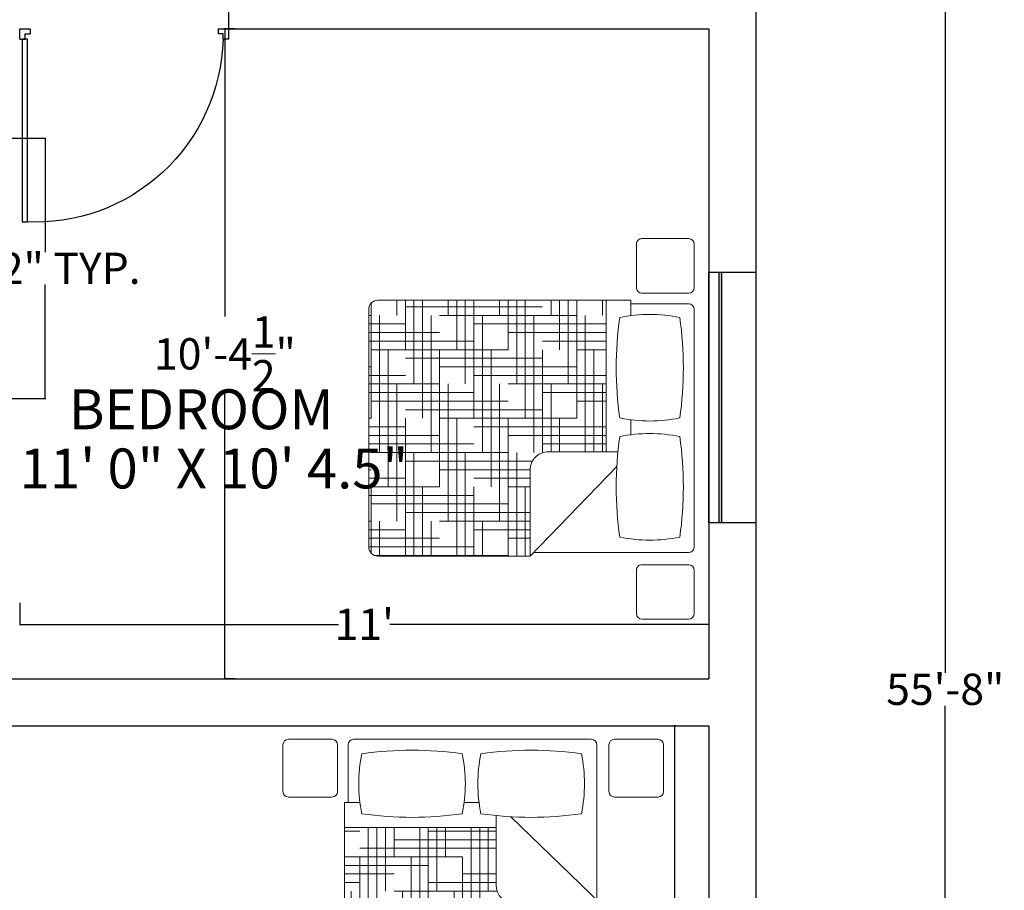
# Model space of a CAD drawing. Units: inches. Extents: x -113 to 5399, y -1393 to 3302.
# Tile 29 of 40: x 3982 to 4170, y 189 to 356. Entities that reach past the tile are written whole.
import ezdxf

# ---------------------------------------------------------------- set-up
doc = ezdxf.new("R2010")
doc.units = ezdxf.units.IN
doc.header["$MEASUREMENT"] = 0
for name, color, linetype, lineweight in [('A-ANNO-DIMS', 254, 'Continuous', 18), ('A-AREA-IDEN', 4, 'Continuous', 18), ('doors', 2, 'Continuous', 25), ('furniture', 131, 'Continuous', 18), ('walls', 1, 'Continuous', 25), ('windows', 3, 'Continuous', 25)]:
    doc.layers.add(name, color=color, linetype=linetype, lineweight=lineweight)
doc.styles.get("Standard").update_dxf_attribs({"font": 'arial.ttf'})
doc.dimstyles.get("Standard").update_dxf_attribs({"dimtxt": 6, "dimasz": 0.18, "dimexe": 0.18, "dimexo": 0.0625, "dimgap": 0.09, "dimtad": 0, "dimtih": 1, "dimtoh": 1, "dimdec": 1, "dimzin": 0, "dimdsep": 46, "dimlunit": 4, "dimtxsty": 'Standard', "dimblk": 'ARCHTICK', "dimcen": 0.09, "dimadec": 0, "dimazin": 0, "dimtfac": 1, "dimtdec": 1, "dimtofl": 0, "dimtmove": 0, "dimatfit": 3, "dimfxl": 1, "dimtolj": 1, "dimtzin": 0, "dimarcsym": 0})

# ---------------------------------------------------------------- blocks, each defined once
blk = doc.blocks.new('*X4')
at = {"color": 0}
for p, q in [((4.3594, 18.5625), (4.3594, 18.6457)), ((4.5, 18), (4.5, 18.6457)), ((4.5469, 18.1875), (4.5469, 18.6457)), ((4.5938, 18.375), (4.5938, 18.6457)), ((4.6406, 18.5625), (4.6406, 18.6457)), ((4.7812, 18), (4.7812, 18.6457)), ((4.8281, 18.1875), (4.8281, 18.6457)), ((4.875, 18.375), (4.875, 18.6457)), ((4.9219, 18.5625), (4.9219, 18.6457)), ((5.0625, 18), (5.0625, 18.6457)), ((5.1094, 18.1875), (5.1094, 18.6457)), ((5.1562, 18.375), (5.1562, 18.6457)), ((5.2031, 18.5625), (5.2031, 18.6457)), ((5.3438, 18), (5.3438, 18.6457)), ((5.3906, 18.1875), (5.3906, 18.6457)), ((5.4375, 18.375), (5.4375, 18.6457)), ((5.4844, 18.5625), (5.4844, 18.6457)), ((4.6875, 18.6094), (5.4375, 18.6094)), ((5.625, 18), (5.625, 18.6287)), ((4.4531, 17.8169), (4.4531, 18.5625)), ((4.5, 18.5625), (5.25, 18.5625)), ((4.7344, 17.8125), (4.7344, 18.5625)), ((5.0156, 17.8125), (5.0156, 18.5625)), ((5.2969, 17.8125), (5.2969, 18.5625)), ((5.5781, 17.8125), (5.5781, 18.5625)), ((5.625, 18.5625), (5.6375, 18.5625)), ((4.3395, 18.5156), (5.0625, 18.5156)), ((5.4375, 18.5156), (5.6375, 18.5156)), ((4.3395, 18.4688), (4.875, 18.4688)), ((4.3395, 18.4219), (4.6875, 18.4219)), ((5.0625, 18.4219), (5.6375, 18.4219)), ((5.25, 18.4688), (5.6375, 18.4688)), ((4.3395, 18.375), (4.5, 18.375)), ((4.4062, 17.8169), (4.4062, 18.375)), ((4.6875, 17.8114), (4.6875, 18.375)), ((4.875, 18.375), (5.625, 18.375)), ((4.9688, 17.625), (4.9688, 18.375)), ((5.25, 17.625), (5.25, 18.375)), ((5.5312, 17.625), (5.5312, 18.375)), ((4.6875, 18.3281), (5.4375, 18.3281)), ((4.5, 18.2812), (5.25, 18.2812)), ((5.625, 18.2812), (5.6375, 18.2812)), ((4.3395, 18.2344), (5.0625, 18.2344)), ((5.4375, 18.2344), (5.6375, 18.2344)), ((4.3395, 18.1875), (4.875, 18.1875)), ((4.3594, 17.8169), (4.3594, 18.1875)), ((4.6406, 17.8169), (4.6406, 18.1875)), ((4.9219, 17.4375), (4.9219, 18.1875)), ((5.2031, 17.4375), (5.2031, 18.1875)), ((5.25, 18.1875), (5.6375, 18.1875)), ((5.4844, 17.4375), (5.4844, 18.1875)), ((4.3395, 18.1406), (4.6875, 18.1406)), ((5.0625, 18.1406), (5.6375, 18.1406)), ((4.3395, 18.0938), (4.5, 18.0938)), ((4.6875, 18.0469), (5.4375, 18.0469)), ((4.875, 18.0938), (5.625, 18.0938)), ((4.5, 18), (5.25, 18)), ((4.5938, 17.8169), (4.5938, 18)), ((4.875, 17.25), (4.875, 18)), ((5.1562, 17.25), (5.1562, 18)), ((5.4375, 17.25), (5.4375, 18)), ((5.625, 18), (5.6375, 18)), ((4.3395, 17.9531), (5.0625, 17.9531)), ((5.4375, 17.9531), (5.6375, 17.9531)), ((4.3395, 17.9062), (4.875, 17.9062)), ((5.25, 17.9062), (5.6375, 17.9062)), ((4.3395, 17.8594), (4.6875, 17.8594)), ((5.0625, 17.8594), (5.6375, 17.8594)), ((4.8281, 17.2457), (4.8281, 17.8125)), ((4.875, 17.8125), (5.625, 17.8125)), ((5.1094, 17.2457), (5.1094, 17.8125)), ((5.3906, 17.2457), (5.3906, 17.8125)), ((4.7421, 17.7656), (5.4375, 17.7656)), ((4.7548, 17.7188), (5.25, 17.7188)), ((5.625, 17.7188), (5.6375, 17.7188)), ((4.7548, 17.6719), (5.0625, 17.6719)), ((5.4375, 17.6719), (5.6375, 17.6719)), ((4.7548, 17.625), (4.875, 17.625)), ((4.7812, 17.2457), (4.7812, 17.625)), ((5.0625, 17.2457), (5.0625, 17.625)), ((5.25, 17.625), (5.6375, 17.625)), ((5.3438, 17.2457), (5.3438, 17.625)), ((5.625, 17.2627), (5.625, 17.625)), ((5.0625, 17.5781), (5.6375, 17.5781)), ((4.875, 17.5312), (5.625, 17.5312)), ((4.7548, 17.4844), (5.4375, 17.4844)), ((4.7548, 17.4375), (5.25, 17.4375)), ((5.0156, 17.2457), (5.0156, 17.4375)), ((5.2969, 17.2457), (5.2969, 17.4375)), ((5.5781, 17.2457), (5.5781, 17.4375)), ((5.625, 17.4375), (5.6375, 17.4375)), ((4.7548, 17.3906), (5.0625, 17.3906)), ((4.7548, 17.3438), (4.875, 17.3438)), ((5.25, 17.3438), (5.6375, 17.3438)), ((5.4375, 17.3906), (5.6375, 17.3906)), ((5.0625, 17.2969), (5.6375, 17.2969)), ((4.875, 17.25), (5.6077, 17.25)), ((4.9688, 17.2457), (4.9688, 17.25)), ((5.25, 17.2457), (5.25, 17.25)), ((5.5312, 17.2457), (5.5312, 17.25))]:
    blk.add_line(p, q, dxfattribs=at)
blk = doc.blocks.new('MAT-P01')
for p, q in [((-0.0213, 0.8164), (-0.0213, 0.5605)), ((0.0087, 0.8464), (0.2471, 0.8464)), ((0.2771, 0.8164), (0.2771, 0.5605)), ((0.3437, 0.8164), (0.3437, -0.0316)), ((0.3737, 0.8464), (1.6737, 0.8464)), ((1.7037, 0.8164), (1.7037, 0.5005)), ((1.7622, 0.8164), (1.7622, 0.5605)), ((1.7922, 0.8464), (2.0306, 0.8464)), ((2.0606, 0.8164), (2.0606, 0.5605)), ((0.0087, 0.5305), (0.2471, 0.5305)), ((0.9879, 0.5005), (1.0693, 0.5005)), ((1.6393, 0.5005), (1.7237, 0.5005)), ((1.7237, 0.5005), (1.7237, -0.8836)), ((1.7922, 0.5305), (2.0306, 0.5305)), ((0.8146, 0.423), (0.3237, -0.0509)), ((0.8949, 0.4293), (0.8949, 0.0491)), ((0.8949, 0.3643), (1.7237, 0.3643)), ((0.8949, 0.3643), (0.8949, 0.0491)), ((0.8949, 0.3643), (1.7237, 0.3643)), ((1.7237, 0.3643), (1.7237, -0.8836)), ((0.3237, -0.0509), (0.7949, -0.0509)), ((0.3237, -0.0509), (0.3237, -0.8836)), ((0.3737, -0.9336), (1.6737, -0.9336))]:
    blk.add_line(p, q)
for centre, radius, start, end in [((0.0087, 0.8164), 0.03, 90, 180), ((0.2471, 0.8164), 0.03, 0, 90), ((0.3737, 0.8164), 0.03, 90, 180), ((1.6737, 0.8164), 0.03, 0, 90), ((1.7922, 0.8164), 0.03, 90, 180), ((2.0306, 0.8164), 0.03, 0, 90), ((1.2251, 0.6034), 0.8138, 168.373, 191.627), ((0.7029, -1.1436), 1.9306, 81.8162, 98.1838), ((0.1806, 0.6034), 0.8138, 348.373, 11.627), ((1.8766, 0.6034), 0.8138, 168.373, 191.627), ((1.3543, -1.1436), 1.9306, 81.8162, 98.1838), ((0.8321, 0.6034), 0.8138, 348.373, 11.627), ((0.0087, 0.5605), 0.03, 180, 270), ((0.2471, 0.5605), 0.03, 270, 0), ((1.7922, 0.5605), 0.03, 180, 270), ((2.0306, 0.5605), 0.03, 270, 0), ((0.7029, 2.3504), 1.9306, 261.8162, 278.1838), ((1.3543, 2.3504), 1.9306, 261.8162, 278.1838), ((0.7949, 0.0491), 0.1, 270, 0), ((0.3737, -0.8836), 0.05, 180, 270), ((1.6737, -0.8836), 0.05, 270, 0)]:
    blk.add_arc(centre, radius, start, end)
at = {"rotation": 270}
blk.add_blockref('*X4', (-16.9221, 4.7038), dxfattribs=at)
blk = doc.blocks.new('_ArchTick')
at = {"color": 0, "linetype": 'ByBlock', "const_width": 0.15}
blk.add_lwpolyline([(-0.5, -0.5), (0.5, 0.5)], dxfattribs=at)
blk = doc.blocks.new('*D103')
at = {"layer": 'A-ANNO-DIMS', "color": 0, "lineweight": -2, "transparency": 16777216}
for p, q in [((4107.42, 220.28), (4106.96, 220.28)), ((4107.14, 220.28), (4107.14, 158.93)), ((4107.14, 91.28), (4107.14, 152.62)), ((4107.42, 91.28), (4106.96, 91.28))]:
    blk.add_line(p, q, dxfattribs=at)
at = {"layer": 'Defpoints', "color": 0, "transparency": 16777216}
for p in [(4107.48, 220.28), (4107.14, 91.28), (4107.48, 91.28)]:
    blk.add_point(p, dxfattribs=at)
at = {"layer": 'A-ANNO-DIMS', "color": 0, "lineweight": -2, "transparency": 16777216, "xscale": 0.18, "yscale": 0.18, "zscale": 0.18}
for p, rotation in [((4107.14, 220.28), 90), ((4107.14, 91.28), 270)]:
    blk.add_blockref('_ArchTick', p, dxfattribs=dict(at, rotation=rotation))
at = {"layer": 'A-ANNO-DIMS', "color": 0, "transparency": 16777216, "insert": (4107.14, 155.78), "char_height": 6, "attachment_point": 5}
blk.add_mtext('\\A1;10\'-9"', dxfattribs=at)
blk = doc.blocks.new('*D121')
at = {"layer": 'A-ANNO-DIMS', "color": 0, "lineweight": -2, "transparency": 16777216}
for p, q in [((4023.01, 353.78), (4020.86, 353.78)), ((4021.04, 353.78), (4021.04, 298.69)), ((4021.04, 229.28), (4021.04, 284.36)), ((4023.01, 229.28), (4020.86, 229.28))]:
    blk.add_line(p, q, dxfattribs=at)
at = {"layer": 'Defpoints', "color": 0, "transparency": 16777216}
for p in [(4023.07, 353.78), (4021.04, 229.28), (4023.07, 229.28)]:
    blk.add_point(p, dxfattribs=at)
at = {"layer": 'A-ANNO-DIMS', "color": 0, "lineweight": -2, "transparency": 16777216, "xscale": 0.18, "yscale": 0.18, "zscale": 0.18}
for p, rotation in [((4021.04, 353.78), 90), ((4021.04, 229.28), 270)]:
    blk.add_blockref('_ArchTick', p, dxfattribs=dict(at, rotation=rotation))
at = {"layer": 'A-ANNO-DIMS', "color": 0, "transparency": 16777216, "insert": (4021.04, 291.53), "char_height": 6, "attachment_point": 5}
blk.add_mtext('\\A1;10\'-4{\\H1x;\\S1/2;}"', dxfattribs=at)
blk = doc.blocks.new('*D122')
at = {"layer": 'A-ANNO-DIMS', "color": 0, "lineweight": -2, "transparency": 16777216}
for p, q in [((3981.73, 243.83), (3981.73, 239.54)), ((4113.73, 243.83), (4113.73, 239.54)), ((3981.73, 239.72), (4042.83, 239.72)), ((4113.73, 239.72), (4052.63, 239.72))]:
    blk.add_line(p, q, dxfattribs=at)
at = {"layer": 'Defpoints', "color": 0, "transparency": 16777216}
for p in [(3981.73, 243.89), (4113.73, 243.89), (4113.73, 239.72)]:
    blk.add_point(p, dxfattribs=at)
at = {"layer": 'A-ANNO-DIMS', "color": 0, "lineweight": -2, "transparency": 16777216, "xscale": 0.18, "yscale": 0.18, "zscale": 0.18, "rotation": 180}
blk.add_blockref('_ArchTick', (3981.73, 239.72), dxfattribs=at)
at = {"layer": 'A-ANNO-DIMS', "color": 0, "lineweight": -2, "transparency": 16777216, "xscale": 0.18, "yscale": 0.18, "zscale": 0.18}
blk.add_blockref('_ArchTick', (4113.73, 239.72), dxfattribs=at)
at = {"layer": 'A-ANNO-DIMS', "color": 0, "transparency": 16777216, "insert": (4047.73, 239.72), "char_height": 6, "attachment_point": 5}
blk.add_mtext("\\A1;11'", dxfattribs=at)
blk = doc.blocks.new('WIN-PLAN-48IN')
h = blk.add_hatch(color=256)
h.dxf.hatch_style = 1
h.paths.add_polyline_path([(48, 2.5), (0, 2.5), (0, 2), (48, 2)])
for p, q in [((0, 9), (48, 9)), ((0, 0), (0, 9)), ((48, 9), (48, 0)), ((48, 2.5), (0, 2.5)), ((48, 2), (0, 2)), ((48, 0), (0, 0))]:
    blk.add_line(p, q)
blk = doc.blocks.new('DOOR-SINGLE-36IN-PLAN')
for p, q in [((0.5, 2), (0.5, 36.98)), ((0.5, 36.98), (1.5, 36.98)), ((1.5, 36.98), (1.5, 2)), ((0, 2), (0, 0)), ((0, 2), (1.04, 2)), ((1.5, 2), (0.5, 2)), ((1.04, 2), (1.04, 0.98)), ((40, 2), (38.96, 2)), ((38.96, 2), (38.96, 0.98)), ((40, 0), (40, 2)), ((1.04, 0.98), (2, 0.98)), ((2, 0), (2, 0.98)), ((38.96, 0.98), (38, 0.98)), ((38, 0), (38, 0.98)), ((0, 0), (2, 0)), ((0, 0), (2, 0)), ((38, 0), (40, 0))]:
    blk.add_line(p, q)
blk.add_arc((2.94, 0.99), 36.04, 1.6003, 93.0893)
blk = doc.blocks.new('*D186')
at = {"layer": 'A-ANNO-DIMS', "color": 0, "lineweight": -2, "transparency": 16777216}
for p, q in [((3974.01, 332.87), (3986.76, 332.87)), ((3986.58, 332.87), (3986.58, 311.03)), ((3986.58, 282.98), (3986.58, 304.82)), ((3974.01, 282.98), (3986.76, 282.98))]:
    blk.add_line(p, q, dxfattribs=at)
at = {"layer": 'Defpoints', "color": 0, "transparency": 16777216}
for p in [(3973.94, 332.87), (3986.58, 332.87), (3973.94, 282.98)]:
    blk.add_point(p, dxfattribs=at)
at = {"layer": 'A-ANNO-DIMS', "color": 0, "lineweight": -2, "transparency": 16777216, "xscale": 0.18, "yscale": 0.18, "zscale": 0.18}
for p, rotation in [((3986.58, 332.87), 90), ((3986.58, 282.98), 270)]:
    blk.add_blockref('_ArchTick', p, dxfattribs=dict(at, rotation=rotation))
at = {"layer": 'A-ANNO-DIMS', "color": 0, "transparency": 16777216, "insert": (3986.58, 307.92), "char_height": 6, "attachment_point": 5}
blk.add_mtext('\\A1;4\'-2" TYP.', dxfattribs=at)
blk = doc.blocks.new('*D210')
at = {"layer": 'A-ANNO-DIMS', "color": 0, "lineweight": -2, "transparency": 16777216}
for p, q in [((3839.79, 561.28), (4159.21, 561.28)), ((4159.03, 561.28), (4159.03, 230.43)), ((4159.03, -106.72), (4159.03, 224.12)), ((3839.79, -106.72), (4159.21, -106.72))]:
    blk.add_line(p, q, dxfattribs=at)
at = {"layer": 'Defpoints', "color": 0, "transparency": 16777216}
for p in [(3839.73, 561.28), (4159.03, 561.28), (3839.73, -106.72)]:
    blk.add_point(p, dxfattribs=at)
at = {"layer": 'A-ANNO-DIMS', "color": 0, "lineweight": -2, "transparency": 16777216, "xscale": 0.18, "yscale": 0.18, "zscale": 0.18}
for p, rotation in [((4159.03, 561.28), 90), ((4159.03, -106.72), 270)]:
    blk.add_blockref('_ArchTick', p, dxfattribs=dict(at, rotation=rotation))
at = {"layer": 'A-ANNO-DIMS', "color": 0, "transparency": 16777216, "insert": (4159.03, 227.28), "char_height": 6, "attachment_point": 5}
blk.add_mtext('\\A1;55\'-8"', dxfattribs=at)

msp = doc.modelspace()

# ---------------------------------------------------------------- linework, layer by layer
at = {"layer": 'walls'}
for p, q in [((4122.73, 549.78), (4122.73, -100.22)), ((4021.73, 382.78), (4021.73, 353.78)), ((4021.73, 353.78), (4113.73, 353.78)), ((4113.73, 353.78), (4113.73, 229.28)), ((3964.73, 229.28), (4113.73, 229.28)), ((3964.73, 220.28), (4113.73, 220.28)), ((4113.73, 220.28), (4113.73, 95.78))]:
    msp.add_line(p, q, dxfattribs=at)

# ---------------------------------------------------------------- block references
at = {"layer": 'doors', "extrusion": (0, 0, -1), "zscale": -1, "rotation": 180}
msp.add_blockref('DOOR-SINGLE-36IN-PLAN', (-3981.73, 353.78), dxfattribs=at)
at = {"layer": 'furniture', "xscale": -35.02364872074636, "yscale": 35.02364872074636, "zscale": 35.02364872074636, "rotation": 270}
msp.add_blockref('MAT-P01', (4081.3, 241.44), dxfattribs=at)
at = {"layer": 'furniture', "xscale": -35.02364872074636, "yscale": 35.02364872074636, "zscale": 35.02364872074636}
msp.add_blockref('MAT-P01', (4104.32, 188.05), dxfattribs=at)
at = {"layer": 'windows', "rotation": 270.0000000000005}
msp.add_blockref('WIN-PLAN-48IN', (4113.73, 307.19), dxfattribs=at)

# ---------------------------------------------------------------- texts
at = {"layer": 'A-AREA-IDEN'}
for s, height, p in [('BEDROOM', 7.647, (3991.12, 277.09)), ('11\' 0" X 10\' 4.5"', 7.6473, (3981.73, 265.75))]:
    msp.add_text(s, height=height, dxfattribs=at).set_placement(p)

# ---------------------------------------------------------------- dimensions: what is measured, and where the dimension line sits
at = {"layer": 'A-ANNO-DIMS'}
for base, p1, p2, override, picture, middle in [((4159.03, 561.28), (3839.73, -106.72), (3839.73, 561.28), {"dimdec": 1, "dimlfac": 1, "dimrnd": 0, "dimzin": 1, "dimdsep": 46, "dimlunit": 4, "dimfrac": 2}, '*D210', (4159.03, 227.28)), ((4021.04, 229.28), (4023.07, 353.78), (4023.07, 229.28), {"dimclrd": 0, "dimclre": 0, "dimclrt": 0}, '*D121', (4021.04, 291.53)), ((4107.14, 91.28), (4107.48, 220.28), (4107.48, 91.28), {"dimclrd": 0, "dimclre": 0, "dimclrt": 0}, '*D103', (4107.14, 155.78))]:
    dim = msp.add_linear_dim(base=base, p1=p1, p2=p2, angle=90, dimstyle='Standard', override=override, dxfattribs=at)
    dim.commit()
    dim.dimension.update_dxf_attribs({"geometry": picture, "text_midpoint": middle})
dim = msp.add_linear_dim(base=(3986.58, 332.87), p1=(3973.94, 282.98), p2=(3973.94, 332.87), angle=90, text='<> TYP.', dimstyle='Standard', override={"dimdec": 1, "dimlfac": 1, "dimrnd": 0, "dimzin": 1, "dimdsep": 46, "dimlunit": 4, "dimfrac": 2}, dxfattribs=at)
dim.commit()
dim.dimension.update_dxf_attribs({"geometry": '*D186', "text_midpoint": (3986.58, 307.92)})
dim = msp.add_linear_dim(base=(4113.73, 239.72), p1=(3981.73, 243.89), p2=(4113.73, 243.89), dimstyle='Standard', override={"dimclrd": 0, "dimclre": 0, "dimclrt": 0}, dxfattribs=at)
dim.commit()
dim.dimension.update_dxf_attribs({"geometry": '*D122', "text_midpoint": (4047.73, 239.72)})

doc.saveas('drawing.dxf')
